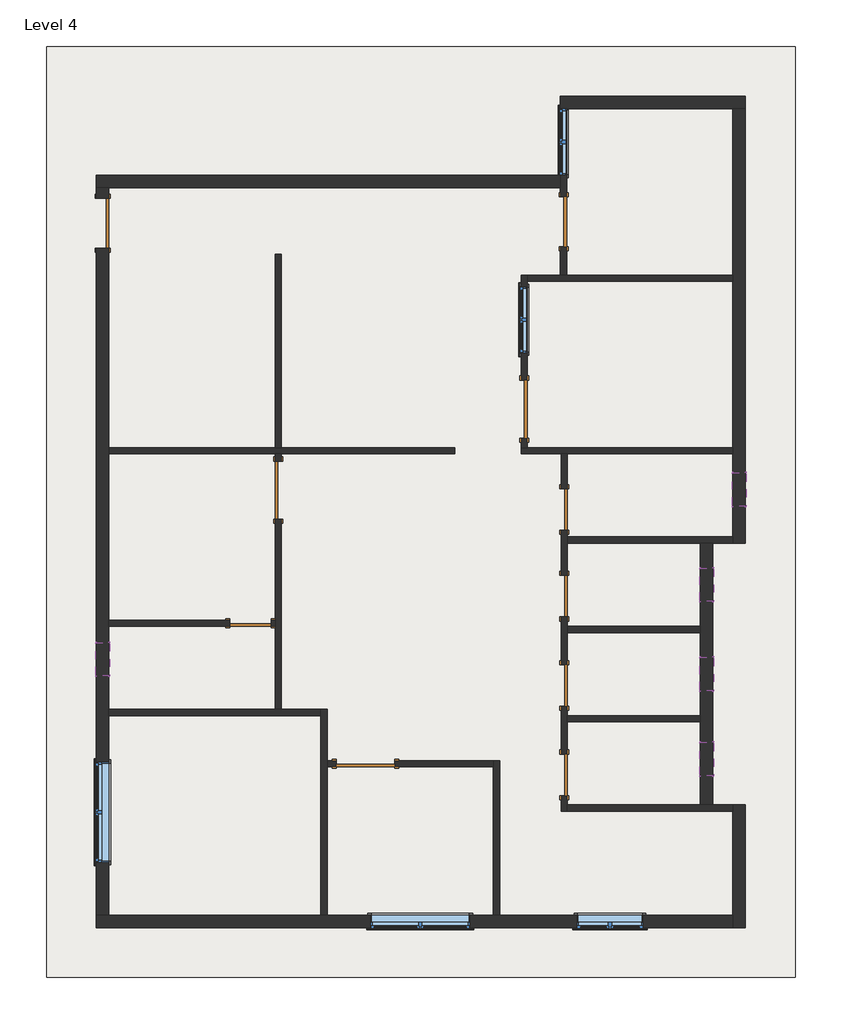
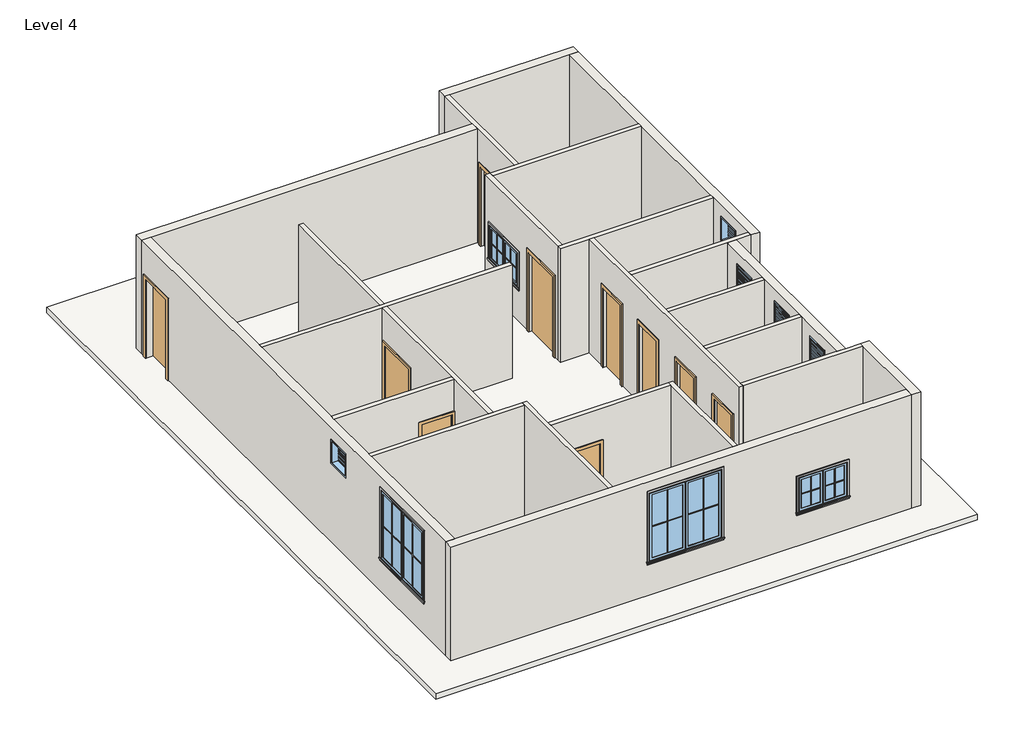
# One storey, incomplete: 23 walls, 20 proxies, 10 doors, 10 windows, 1 roof.
# Revit data of these elements (continued)
# Elements 48, 49, 50, 51, 52, 53, 54 (IfcWall, "WALL 9\"") (continued)
#   Base Offset = 0' - 0"
#   Unconnected Height = 10' - 0"
#   wall height = 10' - 0"
#   Phase Created = New Construction
#   Base Constraint = Level 4
#   Materials on its faces: "Default Wall", "Wood - Stained"
# Element 55 (IfcWindow, "Window-Casement-Double : WIN 4'")
#   Mark = "33"
#   Window Inset = 0' - 0"
#   Interior Wall Closure = 0' - 2 1/4"
#   Frame Extension = 0' - 0 1/4"
#   Exterior Wall Closure = 0' - 1 1/4"
#   Interior Trim Visibility = yes
#   Exterior Trim Visibility = yes
#   Phase Created = New Construction
#   Materials on its faces: "Wood - Stained", "Glass", "Clad - White"
# Element 56 (IfcWindow, "Window-Casement-Double : WIN 4'")
#   Mark = "34"
#   Window Inset = 0' - 0"
#   Interior Wall Closure = 0' - 2 1/4"
#   Frame Extension = 0' - 0 1/4"
#   Exterior Wall Closure = 0' - 1 1/4"
#   Interior Trim Visibility = yes
#   Exterior Trim Visibility = yes
#   Phase Created = New Construction
#   Materials on its faces: "Wood - Stained", "Glass", "Clad - White"
# Element 57 (IfcWindow, "Window-Casement-Double : WIN 4'")
#   Mark = "35"
#   Window Inset = 0' - 0"
#   Interior Wall Closure = 0' - 2 1/4"
#   Frame Extension = 0' - 0 1/4"
#   Exterior Wall Closure = 0' - 1 1/4"
#   Interior Trim Visibility = yes
#   Exterior Trim Visibility = yes
#   Phase Created = New Construction
#   Materials on its faces: "Wood - Stained", "Glass", "Clad - White"
# Element 58 (IfcWindow, "Window-Casement-Double : WIN 6'")
#   Mark = "31"
#   Window Inset = 0' - 0"
#   Interior Wall Closure = 0' - 2 1/4"
#   Frame Extension = 0' - 0 1/4"
#   Exterior Wall Closure = 0' - 1 1/4"
#   Interior Trim Visibility = yes
#   Exterior Trim Visibility = yes
#   Phase Created = New Construction
#   Materials on its faces: "Wood - Stained", "Glass", "Clad - White"
# Element 59 (IfcWindow, "Window-Casement-Double : WIN 6'")
#   Mark = "32"
#   Window Inset = 0' - 0"
#   Interior Wall Closure = 0' - 2 1/4"
#   Frame Extension = 0' - 0 1/4"
#   Exterior Wall Closure = 0' - 1 1/4"
#   Interior Trim Visibility = yes
#   Exterior Trim Visibility = yes
#   Phase Created = New Construction
#   Materials on its faces: "Wood - Stained", "Glass", "Clad - White"
# Element 60 (IfcWindow, "Window-Louvers : 24\" x 24\"")
#   Mark = "36"
#   Blade Width = 1' - 10 1/2"
#   Phase Created = New Construction
#   Materials on its faces: "Birch"
# Element 61 (IfcWindow, "Window-Louvers : 24\" x 24\"")
#   Mark = "37"
#   Blade Width = 1' - 10 1/2"
#   Phase Created = New Construction
#   Materials on its faces: "Birch"
# Element 62 (IfcWindow, "Window-Louvers : 24\" x 24\"")
#   Mark = "38"
#   Blade Width = 1' - 10 1/2"
#   Phase Created = New Construction
#   Materials on its faces: "Birch"
# Element 63 (IfcWindow, "Window-Louvers : 24\" x 24\"")
#   Mark = "39"
#   Blade Width = 1' - 10 1/2"
#   Phase Created = New Construction
#   Materials on its faces: "Birch"
# Element 64 (IfcWindow, "Window-Louvers : 24\" x 24\"")
#   Mark = "40"
#   Blade Width = 1' - 10 1/2"
#   Phase Created = New Construction
#   Materials on its faces: "Birch"
# Materials
#   "Door - Panel": class "Wood", colour RGB 210 159 95, transparency 0, Cost = 0
#   "Door - Frame": colour RGB 118 70 51, transparency 0, Cost = 0
#   "Wood - Stained": class "Wood", colour RGB 224 178 126, transparency 0, Cost = 0
#   "Glass": class "Glass", colour RGB 0 128 192, transparency 0.75, Description = "Soda Lime Glass", Cost = 0
#   "Clad - White": class "Wood", colour RGB 242 242 238, transparency 0, Cost = 0
#   "Birch": class "Wood", colour RGB 224 178 126, transparency 0, Description = "Betula Alleghaniensis", Cost = 0
#   "Default Roof": colour RGB 88 101 114, transparency 0, Cost = 0
#   "Cherry": class "Wood", colour RGB 226 177 128, transparency 0, Description = "Prunus Serotina", Cost = 0
#   "Wood Planks": class "Wood", colour RGB 193 160 115, transparency 0, Description = "Physical material.", Cost = 0
#   "Default Wall": colour RGB 128 128 128, transparency 0, Cost = 0
